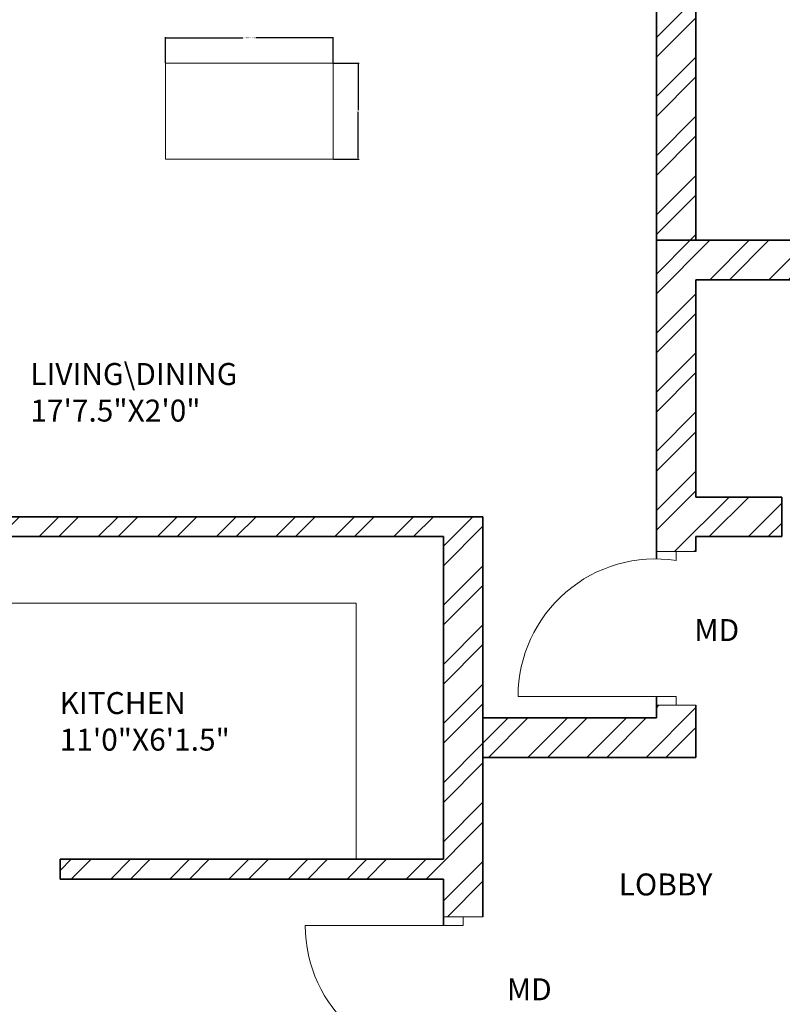
# Model space of a CAD drawing. Units: inches. Extents: x 2120 to 4013, y 1390 to 3019.
# Tile 32 of 59: x 2484 to 2657, y 1964 to 2188. Entities that reach past the tile are written whole.
import ezdxf

# ---------------------------------------------------------------- set-up
doc = ezdxf.new("R2010")
doc.units = ezdxf.units.IN
for name, color, linetype, lineweight in [('A-ANNO-DIMS', 2, 'Continuous', 18), ('A-ANNO-TEXT', 7, 'Continuous', 18), ('A-AREA-IDEN', 7, 'Continuous', 18), ('A-DOOR', 3, 'Continuous', 18), ('A-FLOR-CASE', 8, 'Continuous', 18), ('A-FURN', 8, 'Continuous', 13), ('A-WALL', 7, 'Continuous', 35), ('A-WALL-PATT', 252, 'Continuous', 13)]:
    doc.layers.add(name, color=color, linetype=linetype, lineweight=lineweight)
doc.styles.get("Standard").update_dxf_attribs({"font": 'arial.ttf'})
doc.dimstyles.get("Standard").update_dxf_attribs({"dimtxt": 0.18, "dimasz": 0.18, "dimexe": 0.18, "dimexo": 0.0625, "dimgap": 0.09, "dimtad": 0, "dimtih": 1, "dimtoh": 1, "dimdec": 4, "dimzin": 0, "dimdsep": 46, "dimtxsty": 'Standard', "dimcen": 0.09, "dimadec": 0, "dimazin": 0, "dimtfac": 1, "dimtdec": 4, "dimtofl": 0, "dimtmove": 0, "dimatfit": 3, "dimfxl": 1, "dimtolj": 1, "dimtzin": 0, "dimarcsym": 0})

# ---------------------------------------------------------------- blocks, each defined once
blk = doc.blocks.new('DOOR-SWING-36IN-98p95DEG')
for p, q in [((31.5, 34.77), (40.5, 34.77)), ((40.5, 34.77), (36, 34.77)), ((36, 34.77), (36, 32.77)), ((36, 32.77), (0, 32.77)), ((31.5, 0), (40.5, 0)), ((36, 0), (36, 2)), ((40.5, 0), (36, 0))]:
    blk.add_line(p, q)
blk.add_arc((31.15, 32.77), 31.15, 180, 278.9496)
blk = doc.blocks.new('DOOR-SWING-36IN-98p61DEG')
for p, q in [((40.5, 34.96), (31.5, 34.96)), ((31.5, 34.96), (36, 34.96)), ((36, 34.96), (36, 32.96)), ((36, 2), (0, 2)), ((31.5, 0), (40.5, 0)), ((36, 0), (36, 2)), ((40.5, 0), (36, 0))]:
    blk.add_line(p, q)
blk.add_arc((31.31, 2), 31.31, 81.386, 180)
blk = doc.blocks.new('TABLE-COFFEE')
blk.add_lwpolyline([(0, 38.19), (21.88, 38.19), (21.88, 0), (0, 0)], close=True)
blk = doc.blocks.new('*D77')
at = {"layer": 'A-ANNO-DIMS', "color": 0, "lineweight": -2, "transparency": 16777216}
for p, q in [((2516.9, 2178.46), (2516.9, 2184.3)), ((2517.08, 2184.12), (2534.49, 2184.12)), ((2554.91, 2184.12), (2537.5, 2184.12)), ((2555.09, 2178.46), (2555.09, 2184.3))]:
    blk.add_line(p, q, dxfattribs=at)
at = {"layer": 'A-ANNO-DIMS', "color": 0, "transparency": 16777216}
for points in [[(2517.08, 2184.15), (2517.08, 2184.09), (2516.9, 2184.12)], [(2554.91, 2184.15), (2554.91, 2184.09), (2555.09, 2184.12)]]:
    blk.add_solid(points, dxfattribs=at)
at = {"layer": 'Defpoints', "color": 0, "transparency": 16777216}
for p in [(2516.9, 2184.12), (2516.9, 2178.4), (2555.09, 2178.4)]:
    blk.add_point(p, dxfattribs=at)
at = {"layer": 'A-ANNO-DIMS', "color": 0, "transparency": 16777216, "insert": (2535.99, 2184.12), "char_height": 0.18, "attachment_point": 5}
blk.add_mtext('\\A1;COFFEE TABLE 38 TYP.', dxfattribs=at)
blk = doc.blocks.new('*D78')
at = {"layer": 'A-ANNO-DIMS', "color": 0, "lineweight": -2, "transparency": 16777216}
for p, q in [((2555.15, 2178.4), (2561, 2178.4)), ((2560.82, 2178.22), (2560.82, 2167.64)), ((2560.82, 2156.7), (2560.82, 2167.28)), ((2555.15, 2156.52), (2561, 2156.52))]:
    blk.add_line(p, q, dxfattribs=at)
at = {"layer": 'A-ANNO-DIMS', "color": 0, "transparency": 16777216}
for points in [[(2560.79, 2178.22), (2560.85, 2178.22), (2560.82, 2178.4)], [(2560.79, 2156.7), (2560.85, 2156.7), (2560.82, 2156.52)]]:
    blk.add_solid(points, dxfattribs=at)
at = {"layer": 'Defpoints', "color": 0, "transparency": 16777216}
for p in [(2555.09, 2178.4), (2560.82, 2178.4), (2555.09, 2156.52)]:
    blk.add_point(p, dxfattribs=at)
at = {"layer": 'A-ANNO-DIMS', "color": 0, "transparency": 16777216, "insert": (2560.82, 2167.46), "char_height": 0.18, "attachment_point": 5}
blk.add_mtext('\\A1;22 TYP.', dxfattribs=at)

msp = doc.modelspace()

# ---------------------------------------------------------------- hatches: boundary and pattern name
at = {"layer": 'A-WALL-PATT'}
h = msp.add_hatch(dxfattribs=at)
h.set_pattern_fill('ANSI32', color=256)
h.paths.add_polyline_path([(2271.7331, 2343.531), (2283.3788, 2343.531), (2283.3788, 2348.031), (2283.3788, 2352.5306), (2262.7331, 2352.5306), (2262.7331, 2182.638), (2267.2331, 2182.638), (2271.7331, 2182.638), (2271.7331, 2219.031), (2391.7331, 2219.031), (2391.7331, 2214.189), (2393.9831, 2214.189), (2396.2331, 2214.189), (2396.2331, 2219.031), (2420.2331, 2219.031), (2420.2331, 2225.7535), (2417.2197, 2225.7535), (2415.7331, 2225.7535), (2415.7331, 2223.5306), (2271.7331, 2223.5306)])
h.paths.add_polyline_path([(2380.0942, 2352.5306), (2343.3788, 2352.5306), (2343.3788, 2343.531), (2363.2331, 2343.531), (2363.2331, 2288.8489), (2365.4831, 2288.8489), (2367.7331, 2288.8489), (2367.7331, 2343.531), (2380.0942, 2343.531)], flags=17)
h.paths.add_polyline_path([(2432.4339, 2352.5306), (2404.0943, 2352.5306), (2404.0943, 2343.531), (2415.7331, 2343.531), (2415.7331, 2264.0306), (2367.7331, 2264.0306), (2367.7331, 2266.4872), (2363.2331, 2266.4872), (2363.2331, 2259.531), (2367.7331, 2259.531), (2415.7331, 2259.531), (2415.7331, 2255.0658), (2420.2331, 2255.0658), (2420.2331, 2259.531), (2424.5717, 2259.531), (2424.5717, 2261.781), (2424.5717, 2264.0306), (2420.2331, 2264.0306), (2420.2331, 2343.531), (2432.4339, 2343.531)])
h.paths.add_polyline_path([(2508.9115, 2352.5306), (2456.4339, 2352.5306), (2456.4339, 2343.531), (2468.2331, 2343.531), (2468.2331, 2264.0306), (2448.0487, 2264.0306), (2448.0487, 2259.531), (2468.2331, 2259.531), (2468.2331, 2255.5496), (2472.7331, 2255.5496), (2472.7331, 2343.531), (2508.9115, 2343.531)])
h.paths.add_polyline_path([(2637.7331, 2352.5306), (2544.9116, 2352.5306), (2544.9116, 2343.531), (2589.7331, 2343.531), (2633.2331, 2343.531), (2637.7331, 2343.531)])
h.paths.add_polyline_path([(2594.2331, 2343.5306), (2589.7331, 2343.5306), (2589.7331, 2259.5306), (2589.7331, 2252.4915), (2591.9831, 2252.4915), (2594.2331, 2252.4915)])
h.paths.add_polyline_path([(2637.7331, 2223.5306), (2594.2331, 2223.5306), (2594.2331, 2230.1988), (2591.9831, 2230.1988), (2589.7331, 2230.1988), (2589.7331, 2223.5306), (2472.7331, 2223.5306), (2468.2331, 2223.5306), (2468.2331, 2219.031), (2628.7331, 2219.031), (2628.7331, 2138.031), (2637.7331, 2138.031)])
h.paths.add_polyline_path([(3822.6535, 2458.4402), (3874.9468, 2458.4402), (3874.9468, 2476.9866), (3822.6535, 2476.9866)], flags=9)
h.paths.add_polyline_path([(3834.6921, 2781.8174), (3935.9206, 2781.8174), (3935.9206, 2800.3638), (3834.6921, 2800.3638)], flags=9)
h.paths.add_polyline_path([(3832.2843, 2837.9683), (3884.5776, 2837.9683), (3884.5776, 2856.5146), (3832.2843, 2856.5146)], flags=9)
h.paths.add_polyline_path([(3830.9388, 2861.4782), (3956.8958, 2861.4782), (3956.8958, 2880.0245), (3830.9388, 2880.0245)], flags=9)
h.paths.add_polyline_path([(3870.6966, 2352.5752), (3887.9272, 2352.5752), (3887.9272, 2377.3037), (3870.6966, 2377.3037)], flags=9)
h.paths.add_polyline_path([(3289.2701, 2413.161), (3435.2223, 2413.161), (3435.2223, 2450.2538), (3289.2701, 2450.2538)], flags=9)
h.paths.add_polyline_path([(2487.6944, 2414.3601), (2637.8335, 2414.3601), (2637.8335, 2451.4528), (2487.6944, 2451.4528)], flags=9)
h.paths.add_polyline_path([(2567.3724, 1457.9199), (2815.296, 1457.9199), (2815.296, 1495.0127), (2567.3724, 1495.0127)], flags=9)
h.paths.add_polyline_path([(2655.3825, 2093.2363), (2685.9555, 2093.2363), (2685.9555, 2111.8937), (2655.3825, 2111.8937)], flags=9)
h.paths.add_polyline_path([(2543.9218, 1550.6671), (2587.8406, 1550.6671), (2587.8406, 1569.3244), (2543.9218, 1569.3244)], flags=9)
h.paths.add_polyline_path([(2905.1384, 1543.8113), (2949.0572, 1543.8113), (2949.0572, 1562.4686), (2905.1384, 1562.4686)], flags=9)
h.paths.add_polyline_path([(2736.4118, 1702.4736), (2784.2153, 1702.4736), (2784.2153, 1721.1309), (2736.4118, 1721.1309)], flags=9)
h.paths.add_polyline_path([(2912.8666, 1710.4168), (2951.707, 1710.4168), (2951.707, 1729.0741), (2912.8666, 1729.0741)], flags=9)
h.paths.add_polyline_path([(2923.5785, 1763.5038), (2959.7279, 1763.5038), (2959.7279, 1782.1611), (2923.5785, 1782.1611)], flags=9)
h.paths.add_polyline_path([(2925.2114, 1809.6137), (2967.1861, 1809.6137), (2967.1861, 1828.271), (2925.2114, 1828.271)], flags=9)
h.paths.add_polyline_path([(2996.2711, 1878.9003), (2996.2711, 1913.109), (2977.6138, 1913.109), (2977.6138, 1878.9003)], flags=9)
h.paths.add_polyline_path([(2883.0859, 1895.7192), (2927.1855, 1895.7192), (2927.1855, 1914.3766), (2883.0859, 1914.3766)], flags=9)
h.paths.add_polyline_path([(2787.3924, 1810.8013), (2841.0213, 1810.8013), (2841.0213, 1829.4587), (2787.3924, 1829.4587)], flags=9)
h.paths.add_polyline_path([(2775.6399, 2101.7395), (2829.2689, 2101.7395), (2829.2689, 2120.3968), (2775.6399, 2120.3968)], flags=9)
h.paths.add_polyline_path([(2913.0263, 2075.817), (2951.8667, 2075.817), (2951.8667, 2094.4744), (2913.0263, 2094.4744)], flags=9)
h.paths.add_polyline_path([(2929.966, 2133.3669), (2966.1154, 2133.3669), (2966.1154, 2152.0243), (2929.966, 2152.0243)], flags=9)
h.paths.add_polyline_path([(2932.7502, 2182.6088), (2968.8996, 2182.6088), (2968.8996, 2201.2662), (2932.7502, 2201.2662)], flags=9)
h.paths.add_polyline_path([(2996.0681, 2266.3173), (2996.0681, 2300.5261), (2977.4108, 2300.5261), (2977.4108, 2266.3173)], flags=9)
h.paths.add_polyline_path([(2885.1039, 2279.2186), (2929.2035, 2279.2186), (2929.2035, 2297.8759), (2885.1039, 2297.8759)], flags=9)
h.paths.add_polyline_path([(2735.7042, 2218.3197), (2783.5078, 2218.3197), (2783.5078, 2236.9771), (2735.7042, 2236.9771)], flags=9)
h.paths.add_polyline_path([(2635.6049, 2044.0085), (2648.9678, 2044.0085), (2648.9678, 2054.312), (2635.6049, 2054.312)], flags=9)
h.paths.add_polyline_path([(2714.0148, 1923.0473), (2727.3777, 1923.0473), (2727.3777, 1933.3508), (2714.0148, 1933.3508)], flags=9)
h.paths.add_polyline_path([(2709.0345, 1988.1628), (2722.3974, 1988.1628), (2722.3974, 1998.4663), (2709.0345, 1998.4663)], flags=9)
h.paths.add_polyline_path([(2592.8935, 1962.1763), (2606.2564, 1962.1763), (2606.2564, 1972.4799), (2592.8935, 1972.4799)], flags=9)
h.paths.add_polyline_path([(2618.3996, 1985.9724), (2644.1942, 1985.9724), (2644.1942, 1996.2759), (2618.3996, 1996.2759)], flags=9)
h.paths.add_polyline_path([(2601.279, 1920.5869), (2614.6419, 1920.5869), (2614.6419, 1930.8904), (2601.279, 1930.8904)], flags=9)
h.paths.add_polyline_path([(2692.3278, 1932.7645), (2704.5311, 1932.7645), (2704.5311, 1943.0681), (2692.3278, 1943.0681)], flags=9)
h.paths.add_polyline_path([(2311.122, 1672.7318), (2355.0408, 1672.7318), (2355.0408, 1691.3892), (2311.122, 1691.3892)], flags=9)
h.paths.add_polyline_path([(2456.2551, 1632.3198), (2492.4796, 1632.3198), (2492.4796, 1650.9772), (2456.2551, 1650.9772)], flags=9)
h.paths.add_polyline_path([(2401.0766, 1631.4793), (2437.301, 1631.4793), (2437.301, 1650.1367), (2401.0766, 1650.1367)], flags=9)
h.paths.add_polyline_path([(2546.7054, 1700.9235), (2594.509, 1700.9235), (2594.509, 1719.5809), (2546.7054, 1719.5809)], flags=9)
h.paths.add_polyline_path([(2445.4866, 1766.9937), (2497.5261, 1766.9937), (2497.5261, 1785.651), (2445.4866, 1785.651)], flags=9)
h.paths.add_polyline_path([(2287.9992, 1739.7675), (2326.8396, 1739.7675), (2326.8396, 1758.4248), (2287.9992, 1758.4248)], flags=9)
h.paths.add_polyline_path([(2458.5279, 1924.7607), (2510.5675, 1924.7607), (2510.5675, 1943.4181), (2458.5279, 1943.4181)], flags=9)
h.paths.add_polyline_path([(2309.2811, 1902.7642), (2345.4305, 1902.7642), (2345.4305, 1921.4215), (2309.2811, 1921.4215)], flags=9)
h.paths.add_polyline_path([(2490.7554, 2018.9392), (2530.7896, 2018.9392), (2530.7896, 2037.5965), (2490.7554, 2037.5965)], flags=9)
h.paths.add_polyline_path([(2402.143, 2024.7393), (2438.5414, 2024.7393), (2438.5414, 2043.3966), (2402.143, 2043.3966)], flags=9)
h.paths.add_polyline_path([(2287.856, 1931.7926), (2326.6964, 1931.7926), (2326.6964, 1950.4499), (2287.856, 1950.4499)], flags=9)
h.paths.add_polyline_path([(2281.7979, 2193.5771), (2320.6383, 2193.5771), (2320.6383, 2212.2344), (2281.7979, 2212.2344)], flags=25)
h.paths.add_polyline_path([(2484.0754, 2093.892), (2536.115, 2093.892), (2536.115, 2112.5494), (2484.0754, 2112.5494)], flags=9)
h.paths.add_polyline_path([(2624.7948, 2281.8639), (2624.7948, 2311.4137), (2606.1375, 2311.4137), (2606.1375, 2281.8639)], flags=9)
h.paths.add_polyline_path([(2507.5036, 2290.3639), (2541.934, 2290.3639), (2541.934, 2309.0212), (2507.5036, 2309.0212)], flags=9)
h.paths.add_polyline_path([(2423.1076, 2285.2202), (2459.332, 2285.2202), (2459.332, 2303.8776), (2423.1076, 2303.8776)], flags=9)
h.paths.add_polyline_path([(2374.5467, 2289.6272), (2410.7711, 2289.6272), (2410.7711, 2308.2846), (2374.5467, 2308.2846)], flags=25)
h.paths.add_polyline_path([(2277.4907, 2227.5651), (2316.3311, 2227.5651), (2316.3311, 2246.2224), (2277.4907, 2246.2224)], flags=25)
h.paths.add_polyline_path([(2655.3825, 2093.2367), (2685.9555, 2093.2367), (2685.9555, 2111.894), (2655.3825, 2111.894)], flags=9)
h.paths.add_polyline_path([(2543.9217, 1550.6674), (2587.8406, 1550.6674), (2587.8406, 1569.3247), (2543.9217, 1569.3247)], flags=9)
h.paths.add_polyline_path([(2905.1384, 1543.8116), (2949.0572, 1543.8116), (2949.0572, 1562.4689), (2905.1384, 1562.4689)], flags=9)
h.paths.add_polyline_path([(2736.4118, 1702.4739), (2784.2153, 1702.4739), (2784.2153, 1721.1312), (2736.4118, 1721.1312)], flags=9)
h.paths.add_polyline_path([(2912.8666, 1710.4171), (2951.707, 1710.4171), (2951.707, 1729.0744), (2912.8666, 1729.0744)], flags=9)
h.paths.add_polyline_path([(2923.5785, 1763.5041), (2959.7279, 1763.5041), (2959.7279, 1782.1614), (2923.5785, 1782.1614)], flags=9)
h.paths.add_polyline_path([(2925.2114, 1809.614), (2967.1861, 1809.614), (2967.1861, 1828.2713), (2925.2114, 1828.2713)], flags=9)
h.paths.add_polyline_path([(2996.2711, 1878.9006), (2996.2711, 1913.1094), (2977.6137, 1913.1094), (2977.6137, 1878.9006)], flags=9)
h.paths.add_polyline_path([(2883.0859, 1895.7195), (2927.1855, 1895.7195), (2927.1855, 1914.3769), (2883.0859, 1914.3769)], flags=9)
h.paths.add_polyline_path([(2787.3924, 1810.8016), (2841.0213, 1810.8016), (2841.0213, 1829.459), (2787.3924, 1829.459)], flags=9)
h.paths.add_polyline_path([(2775.6399, 2101.7398), (2829.2688, 2101.7398), (2829.2688, 2120.3971), (2775.6399, 2120.3971)], flags=9)
h.paths.add_polyline_path([(2913.0263, 2075.8173), (2951.8667, 2075.8173), (2951.8667, 2094.4747), (2913.0263, 2094.4747)], flags=9)
h.paths.add_polyline_path([(2929.966, 2133.3672), (2966.1154, 2133.3672), (2966.1154, 2152.0246), (2929.966, 2152.0246)], flags=9)
h.paths.add_polyline_path([(2932.7502, 2182.6091), (2968.8996, 2182.6091), (2968.8996, 2201.2665), (2932.7502, 2201.2665)], flags=9)
h.paths.add_polyline_path([(2996.0681, 2266.3176), (2996.0681, 2300.5264), (2977.4108, 2300.5264), (2977.4108, 2266.3176)], flags=9)
h.paths.add_polyline_path([(2885.1039, 2279.2189), (2929.2035, 2279.2189), (2929.2035, 2297.8762), (2885.1039, 2297.8762)], flags=9)
h.paths.add_polyline_path([(2735.7042, 2218.32), (2783.5078, 2218.32), (2783.5078, 2236.9774), (2735.7042, 2236.9774)], flags=9)
h.paths.add_polyline_path([(2635.6048, 2044.0088), (2648.9677, 2044.0088), (2648.9677, 2054.3123), (2635.6048, 2054.3123)], flags=9)
h.paths.add_polyline_path([(2714.0148, 1923.0476), (2727.3777, 1923.0476), (2727.3777, 1933.3511), (2714.0148, 1933.3511)], flags=9)
h.paths.add_polyline_path([(2709.0345, 1988.1631), (2722.3974, 1988.1631), (2722.3974, 1998.4666), (2709.0345, 1998.4666)], flags=9)
h.paths.add_polyline_path([(2592.8935, 1962.1766), (2606.2564, 1962.1766), (2606.2564, 1972.4802), (2592.8935, 1972.4802)], flags=9)
h.paths.add_polyline_path([(2618.3995, 1985.9727), (2644.1942, 1985.9727), (2644.1942, 1996.2762), (2618.3995, 1996.2762)], flags=9)
h.paths.add_polyline_path([(2601.279, 1920.5872), (2614.6419, 1920.5872), (2614.6419, 1930.8908), (2601.279, 1930.8908)], flags=9)
h.paths.add_polyline_path([(2692.3278, 1932.7648), (2704.5311, 1932.7648), (2704.5311, 1943.0684), (2692.3278, 1943.0684)], flags=9)
h.paths.add_polyline_path([(2311.122, 1672.7321), (2355.0408, 1672.7321), (2355.0408, 1691.3895), (2311.122, 1691.3895)], flags=9)
h.paths.add_polyline_path([(2456.2551, 1632.3201), (2492.4795, 1632.3201), (2492.4795, 1650.9775), (2456.2551, 1650.9775)], flags=9)
h.paths.add_polyline_path([(2401.0766, 1631.4796), (2437.301, 1631.4796), (2437.301, 1650.137), (2401.0766, 1650.137)], flags=9)
h.paths.add_polyline_path([(2546.7054, 1700.9238), (2594.509, 1700.9238), (2594.509, 1719.5812), (2546.7054, 1719.5812)], flags=9)
h.paths.add_polyline_path([(2445.4866, 1766.994), (2497.5261, 1766.994), (2497.5261, 1785.6513), (2445.4866, 1785.6513)], flags=9)
h.paths.add_polyline_path([(2287.9992, 1739.7678), (2326.8396, 1739.7678), (2326.8396, 1758.4251), (2287.9992, 1758.4251)], flags=9)
h.paths.add_polyline_path([(2458.5279, 1924.7611), (2510.5675, 1924.7611), (2510.5675, 1943.4184), (2458.5279, 1943.4184)], flags=9)
h.paths.add_polyline_path([(2309.2811, 1902.7645), (2345.4305, 1902.7645), (2345.4305, 1921.4218), (2309.2811, 1921.4218)], flags=9)
h.paths.add_polyline_path([(2490.7554, 2018.9395), (2530.7895, 2018.9395), (2530.7895, 2037.5968), (2490.7554, 2037.5968)], flags=9)
h.paths.add_polyline_path([(2402.143, 2024.7396), (2438.5413, 2024.7396), (2438.5413, 2043.3969), (2402.143, 2043.3969)], flags=9)
h.paths.add_polyline_path([(2287.856, 1931.7929), (2326.6964, 1931.7929), (2326.6964, 1950.4502), (2287.856, 1950.4502)], flags=9)
h.paths.add_polyline_path([(2281.7979, 2193.5774), (2320.6383, 2193.5774), (2320.6383, 2212.2347), (2281.7979, 2212.2347)], flags=25)
h.paths.add_polyline_path([(2484.0754, 2093.8924), (2536.115, 2093.8924), (2536.115, 2112.5497), (2484.0754, 2112.5497)], flags=9)
h.paths.add_polyline_path([(2624.7948, 2281.8642), (2624.7948, 2311.414), (2606.1374, 2311.414), (2606.1374, 2281.8642)], flags=9)
h.paths.add_polyline_path([(2507.5035, 2290.3642), (2541.934, 2290.3642), (2541.934, 2309.0215), (2507.5035, 2309.0215)], flags=9)
h.paths.add_polyline_path([(2423.1075, 2285.2205), (2459.332, 2285.2205), (2459.332, 2303.8779), (2423.1075, 2303.8779)], flags=9)
h.paths.add_polyline_path([(2374.5467, 2289.6275), (2410.7711, 2289.6275), (2410.7711, 2308.2849), (2374.5467, 2308.2849)], flags=25)
h.paths.add_polyline_path([(2277.4907, 2227.5654), (2316.3311, 2227.5654), (2316.3311, 2246.2227), (2277.4907, 2246.2227)], flags=25)
h = msp.add_hatch(dxfattribs=at)
h.set_pattern_fill('ANSI32', color=256)
h.paths.add_polyline_path([(2271.7331, 1980.389), (2262.7331, 1980.389), (2262.7331, 1912.8434), (2267.2331, 1912.8434), (2271.7331, 1912.8434), (2271.7331, 1922.531), (2351.2331, 1922.531), (2351.2331, 1901.4728), (2355.7331, 1901.4728), (2355.7331, 1922.531), (2357.9815, 1922.531), (2357.9815, 1926.5306), (2271.7331, 1926.5306)])
h.paths.add_polyline_path([(2589.2331, 1949.1622), (2584.7331, 1949.1622), (2580.2331, 1949.1622), (2580.2331, 1874.5306), (2355.7331, 1874.5306), (2355.7331, 1880.1922), (2351.2331, 1880.1922), (2351.2331, 1874.5306), (2271.7331, 1874.5306), (2271.7331, 1888.8431), (2262.7331, 1888.8431), (2262.7331, 1842.2909), (2267.2331, 1842.2909), (2271.7331, 1842.2909), (2271.7331, 1865.531), (2415.7331, 1865.531), (2415.7331, 1779.7286), (2420.2331, 1779.7286), (2420.2331, 1865.531), (2589.2331, 1865.531)])
h.paths.add_polyline_path([(2271.7331, 1782.2906), (2262.7331, 1782.2906), (2262.7331, 1711.4639), (2267.2331, 1711.4639), (2271.7331, 1711.4639), (2271.7331, 1738.031), (2420.2331, 1738.031), (2420.2331, 1742.531), (2420.2331, 1747.3376), (2417.9831, 1747.3376), (2415.7331, 1747.3376), (2415.7331, 1742.5306), (2271.7331, 1742.5306)])
h.paths.add_polyline_path([(2271.7331, 1627.031), (2362.3957, 1627.031), (2362.3957, 1629.281), (2362.3957, 1631.5306), (2271.7331, 1631.5306), (2271.7331, 1675.4636), (2262.7331, 1675.4636), (2262.7331, 1581.531), (2405.3032, 1581.531), (2405.3032, 1586.031), (2405.3032, 1590.5306), (2396.2331, 1590.5306), (2396.2331, 1691.4513), (2418.7206, 1691.4513), (2418.7206, 1695.951), (2396.2331, 1695.951), (2391.7331, 1695.951), (2391.7331, 1631.5306), (2386.7425, 1631.5306), (2386.7425, 1629.2806), (2386.7425, 1627.031), (2391.7331, 1627.031), (2391.7331, 1586.1709), (2271.7331, 1586.1709)])
h.paths.add_polyline_path([(2459.6703, 1590.5306), (2429.3032, 1590.5306), (2429.3032, 1581.531), (2459.6703, 1581.531), (2459.6703, 1586.031)])
h.paths.add_polyline_path([(2501.2331, 1590.531), (2501.2331, 1665.0195), (2498.9831, 1665.0195), (2496.7331, 1665.0195), (2496.7331, 1590.5306), (2483.8201, 1590.5306), (2483.8201, 1590.1579), (2483.6704, 1590.1579), (2483.6704, 1581.531), (2505.0196, 1581.531), (2505.0196, 1583.781), (2505.0196, 1586.0306), (2501.2331, 1586.0306)])
h.paths.add_polyline_path([(2544.1361, 1583.781), (2544.1361, 1586.0306), (2527.1368, 1586.0306), (2527.1368, 1583.7806), (2527.1368, 1581.531), (2544.1361, 1581.531)])
h.paths.add_polyline_path([(3822.6535, 2458.4402), (3874.9468, 2458.4402), (3874.9468, 2476.9866), (3822.6535, 2476.9866)], flags=9)
h.paths.add_polyline_path([(3834.6921, 2781.8174), (3935.9206, 2781.8174), (3935.9206, 2800.3638), (3834.6921, 2800.3638)], flags=9)
h.paths.add_polyline_path([(3832.2843, 2837.9683), (3884.5776, 2837.9683), (3884.5776, 2856.5146), (3832.2843, 2856.5146)], flags=9)
h.paths.add_polyline_path([(3830.9388, 2861.4782), (3956.8958, 2861.4782), (3956.8958, 2880.0245), (3830.9388, 2880.0245)], flags=9)
h.paths.add_polyline_path([(3870.6966, 2352.5752), (3887.9272, 2352.5752), (3887.9272, 2377.3037), (3870.6966, 2377.3037)], flags=9)
h.paths.add_polyline_path([(3289.2701, 2413.161), (3435.2223, 2413.161), (3435.2223, 2450.2538), (3289.2701, 2450.2538)], flags=9)
h.paths.add_polyline_path([(2487.6944, 2414.3601), (2637.8335, 2414.3601), (2637.8335, 2451.4528), (2487.6944, 2451.4528)], flags=9)
h.paths.add_polyline_path([(2567.3724, 1457.9199), (2815.296, 1457.9199), (2815.296, 1495.0127), (2567.3724, 1495.0127)], flags=9)
h.paths.add_polyline_path([(2655.3825, 2093.2363), (2685.9555, 2093.2363), (2685.9555, 2111.8937), (2655.3825, 2111.8937)], flags=9)
h.paths.add_polyline_path([(2543.9218, 1550.6671), (2587.8406, 1550.6671), (2587.8406, 1569.3244), (2543.9218, 1569.3244)], flags=9)
h.paths.add_polyline_path([(2905.1384, 1543.8113), (2949.0572, 1543.8113), (2949.0572, 1562.4686), (2905.1384, 1562.4686)], flags=9)
h.paths.add_polyline_path([(2736.4118, 1702.4736), (2784.2153, 1702.4736), (2784.2153, 1721.1309), (2736.4118, 1721.1309)], flags=9)
h.paths.add_polyline_path([(2912.8666, 1710.4168), (2951.707, 1710.4168), (2951.707, 1729.0741), (2912.8666, 1729.0741)], flags=9)
h.paths.add_polyline_path([(2923.5785, 1763.5038), (2959.7279, 1763.5038), (2959.7279, 1782.1611), (2923.5785, 1782.1611)], flags=9)
h.paths.add_polyline_path([(2925.2114, 1809.6137), (2967.1861, 1809.6137), (2967.1861, 1828.271), (2925.2114, 1828.271)], flags=9)
h.paths.add_polyline_path([(2996.2711, 1878.9003), (2996.2711, 1913.109), (2977.6138, 1913.109), (2977.6138, 1878.9003)], flags=9)
h.paths.add_polyline_path([(2883.0859, 1895.7192), (2927.1855, 1895.7192), (2927.1855, 1914.3766), (2883.0859, 1914.3766)], flags=9)
h.paths.add_polyline_path([(2787.3924, 1810.8013), (2841.0213, 1810.8013), (2841.0213, 1829.4587), (2787.3924, 1829.4587)], flags=9)
h.paths.add_polyline_path([(2775.6399, 2101.7395), (2829.2689, 2101.7395), (2829.2689, 2120.3968), (2775.6399, 2120.3968)], flags=9)
h.paths.add_polyline_path([(2913.0263, 2075.817), (2951.8667, 2075.817), (2951.8667, 2094.4744), (2913.0263, 2094.4744)], flags=9)
h.paths.add_polyline_path([(2929.966, 2133.3669), (2966.1154, 2133.3669), (2966.1154, 2152.0243), (2929.966, 2152.0243)], flags=9)
h.paths.add_polyline_path([(2932.7502, 2182.6088), (2968.8996, 2182.6088), (2968.8996, 2201.2662), (2932.7502, 2201.2662)], flags=9)
h.paths.add_polyline_path([(2996.0681, 2266.3173), (2996.0681, 2300.5261), (2977.4108, 2300.5261), (2977.4108, 2266.3173)], flags=9)
h.paths.add_polyline_path([(2885.1039, 2279.2186), (2929.2035, 2279.2186), (2929.2035, 2297.8759), (2885.1039, 2297.8759)], flags=9)
h.paths.add_polyline_path([(2735.7042, 2218.3197), (2783.5078, 2218.3197), (2783.5078, 2236.9771), (2735.7042, 2236.9771)], flags=9)
h.paths.add_polyline_path([(2635.6049, 2044.0085), (2648.9678, 2044.0085), (2648.9678, 2054.312), (2635.6049, 2054.312)], flags=9)
h.paths.add_polyline_path([(2714.0148, 1923.0473), (2727.3777, 1923.0473), (2727.3777, 1933.3508), (2714.0148, 1933.3508)], flags=9)
h.paths.add_polyline_path([(2709.0345, 1988.1628), (2722.3974, 1988.1628), (2722.3974, 1998.4663), (2709.0345, 1998.4663)], flags=9)
h.paths.add_polyline_path([(2592.8935, 1962.1763), (2606.2564, 1962.1763), (2606.2564, 1972.4799), (2592.8935, 1972.4799)], flags=9)
h.paths.add_polyline_path([(2618.3996, 1985.9724), (2644.1942, 1985.9724), (2644.1942, 1996.2759), (2618.3996, 1996.2759)], flags=9)
h.paths.add_polyline_path([(2601.279, 1920.5869), (2614.6419, 1920.5869), (2614.6419, 1930.8904), (2601.279, 1930.8904)], flags=9)
h.paths.add_polyline_path([(2692.3278, 1932.7645), (2704.5311, 1932.7645), (2704.5311, 1943.0681), (2692.3278, 1943.0681)], flags=9)
h.paths.add_polyline_path([(2311.122, 1672.7318), (2355.0408, 1672.7318), (2355.0408, 1691.3892), (2311.122, 1691.3892)], flags=25)
h.paths.add_polyline_path([(2456.2551, 1632.3198), (2492.4796, 1632.3198), (2492.4796, 1650.9772), (2456.2551, 1650.9772)], flags=9)
h.paths.add_polyline_path([(2401.0766, 1631.4793), (2437.301, 1631.4793), (2437.301, 1650.1367), (2401.0766, 1650.1367)], flags=9)
h.paths.add_polyline_path([(2546.7054, 1700.9235), (2594.509, 1700.9235), (2594.509, 1719.5809), (2546.7054, 1719.5809)], flags=9)
h.paths.add_polyline_path([(2445.4866, 1766.9937), (2497.5261, 1766.9937), (2497.5261, 1785.651), (2445.4866, 1785.651)], flags=9)
h.paths.add_polyline_path([(2287.9992, 1739.7675), (2326.8396, 1739.7675), (2326.8396, 1758.4248), (2287.9992, 1758.4248)], flags=24)
h.paths.add_polyline_path([(2458.5279, 1924.7607), (2510.5675, 1924.7607), (2510.5675, 1943.4181), (2458.5279, 1943.4181)], flags=25)
h.paths.add_polyline_path([(2309.2811, 1902.7642), (2345.4305, 1902.7642), (2345.4305, 1921.4215), (2309.2811, 1921.4215)], flags=25)
h.paths.add_polyline_path([(2490.7554, 2018.9392), (2530.7896, 2018.9392), (2530.7896, 2037.5965), (2490.7554, 2037.5965)], flags=9)
h.paths.add_polyline_path([(2402.143, 2024.7393), (2438.5414, 2024.7393), (2438.5414, 2043.3966), (2402.143, 2043.3966)], flags=9)
h.paths.add_polyline_path([(2287.856, 1931.7926), (2326.6964, 1931.7926), (2326.6964, 1950.4499), (2287.856, 1950.4499)], flags=25)
h.paths.add_polyline_path([(2281.7979, 2193.5771), (2320.6383, 2193.5771), (2320.6383, 2212.2344), (2281.7979, 2212.2344)], flags=9)
h.paths.add_polyline_path([(2484.0754, 2093.892), (2536.115, 2093.892), (2536.115, 2112.5494), (2484.0754, 2112.5494)], flags=9)
h.paths.add_polyline_path([(2624.7948, 2281.8639), (2624.7948, 2311.4137), (2606.1375, 2311.4137), (2606.1375, 2281.8639)], flags=9)
h.paths.add_polyline_path([(2507.5036, 2290.3639), (2541.934, 2290.3639), (2541.934, 2309.0212), (2507.5036, 2309.0212)], flags=9)
h.paths.add_polyline_path([(2423.1076, 2285.2202), (2459.332, 2285.2202), (2459.332, 2303.8776), (2423.1076, 2303.8776)], flags=9)
h.paths.add_polyline_path([(2374.5467, 2289.6272), (2410.7711, 2289.6272), (2410.7711, 2308.2846), (2374.5467, 2308.2846)], flags=9)
h.paths.add_polyline_path([(2277.4907, 2227.5651), (2316.3311, 2227.5651), (2316.3311, 2246.2224), (2277.4907, 2246.2224)], flags=9)
h.paths.add_polyline_path([(2655.3825, 2093.2367), (2685.9555, 2093.2367), (2685.9555, 2111.894), (2655.3825, 2111.894)], flags=9)
h.paths.add_polyline_path([(2543.9217, 1550.6674), (2587.8406, 1550.6674), (2587.8406, 1569.3247), (2543.9217, 1569.3247)], flags=9)
h.paths.add_polyline_path([(2905.1384, 1543.8116), (2949.0572, 1543.8116), (2949.0572, 1562.4689), (2905.1384, 1562.4689)], flags=9)
h.paths.add_polyline_path([(2736.4118, 1702.4739), (2784.2153, 1702.4739), (2784.2153, 1721.1312), (2736.4118, 1721.1312)], flags=9)
h.paths.add_polyline_path([(2912.8666, 1710.4171), (2951.707, 1710.4171), (2951.707, 1729.0744), (2912.8666, 1729.0744)], flags=9)
h.paths.add_polyline_path([(2923.5785, 1763.5041), (2959.7279, 1763.5041), (2959.7279, 1782.1614), (2923.5785, 1782.1614)], flags=9)
h.paths.add_polyline_path([(2925.2114, 1809.614), (2967.1861, 1809.614), (2967.1861, 1828.2713), (2925.2114, 1828.2713)], flags=9)
h.paths.add_polyline_path([(2996.2711, 1878.9006), (2996.2711, 1913.1094), (2977.6137, 1913.1094), (2977.6137, 1878.9006)], flags=9)
h.paths.add_polyline_path([(2883.0859, 1895.7195), (2927.1855, 1895.7195), (2927.1855, 1914.3769), (2883.0859, 1914.3769)], flags=9)
h.paths.add_polyline_path([(2787.3924, 1810.8016), (2841.0213, 1810.8016), (2841.0213, 1829.459), (2787.3924, 1829.459)], flags=9)
h.paths.add_polyline_path([(2775.6399, 2101.7398), (2829.2688, 2101.7398), (2829.2688, 2120.3971), (2775.6399, 2120.3971)], flags=9)
h.paths.add_polyline_path([(2913.0263, 2075.8173), (2951.8667, 2075.8173), (2951.8667, 2094.4747), (2913.0263, 2094.4747)], flags=9)
h.paths.add_polyline_path([(2929.966, 2133.3672), (2966.1154, 2133.3672), (2966.1154, 2152.0246), (2929.966, 2152.0246)], flags=9)
h.paths.add_polyline_path([(2932.7502, 2182.6091), (2968.8996, 2182.6091), (2968.8996, 2201.2665), (2932.7502, 2201.2665)], flags=9)
h.paths.add_polyline_path([(2996.0681, 2266.3176), (2996.0681, 2300.5264), (2977.4108, 2300.5264), (2977.4108, 2266.3176)], flags=9)
h.paths.add_polyline_path([(2885.1039, 2279.2189), (2929.2035, 2279.2189), (2929.2035, 2297.8762), (2885.1039, 2297.8762)], flags=9)
h.paths.add_polyline_path([(2735.7042, 2218.32), (2783.5078, 2218.32), (2783.5078, 2236.9774), (2735.7042, 2236.9774)], flags=9)
h.paths.add_polyline_path([(2635.6048, 2044.0088), (2648.9677, 2044.0088), (2648.9677, 2054.3123), (2635.6048, 2054.3123)], flags=9)
h.paths.add_polyline_path([(2714.0148, 1923.0476), (2727.3777, 1923.0476), (2727.3777, 1933.3511), (2714.0148, 1933.3511)], flags=9)
h.paths.add_polyline_path([(2709.0345, 1988.1631), (2722.3974, 1988.1631), (2722.3974, 1998.4666), (2709.0345, 1998.4666)], flags=9)
h.paths.add_polyline_path([(2592.8935, 1962.1766), (2606.2564, 1962.1766), (2606.2564, 1972.4802), (2592.8935, 1972.4802)], flags=9)
h.paths.add_polyline_path([(2618.3995, 1985.9727), (2644.1942, 1985.9727), (2644.1942, 1996.2762), (2618.3995, 1996.2762)], flags=9)
h.paths.add_polyline_path([(2601.279, 1920.5872), (2614.6419, 1920.5872), (2614.6419, 1930.8908), (2601.279, 1930.8908)], flags=9)
h.paths.add_polyline_path([(2692.3278, 1932.7648), (2704.5311, 1932.7648), (2704.5311, 1943.0684), (2692.3278, 1943.0684)], flags=9)
h.paths.add_polyline_path([(2311.122, 1672.7321), (2355.0408, 1672.7321), (2355.0408, 1691.3895), (2311.122, 1691.3895)], flags=25)
h.paths.add_polyline_path([(2456.2551, 1632.3201), (2492.4795, 1632.3201), (2492.4795, 1650.9775), (2456.2551, 1650.9775)], flags=9)
h.paths.add_polyline_path([(2401.0766, 1631.4796), (2437.301, 1631.4796), (2437.301, 1650.137), (2401.0766, 1650.137)], flags=9)
h.paths.add_polyline_path([(2546.7054, 1700.9238), (2594.509, 1700.9238), (2594.509, 1719.5812), (2546.7054, 1719.5812)], flags=9)
h.paths.add_polyline_path([(2445.4866, 1766.994), (2497.5261, 1766.994), (2497.5261, 1785.6513), (2445.4866, 1785.6513)], flags=9)
h.paths.add_polyline_path([(2287.9992, 1739.7678), (2326.8396, 1739.7678), (2326.8396, 1758.4251), (2287.9992, 1758.4251)], flags=24)
h.paths.add_polyline_path([(2458.5279, 1924.7611), (2510.5675, 1924.7611), (2510.5675, 1943.4184), (2458.5279, 1943.4184)], flags=25)
h.paths.add_polyline_path([(2309.2811, 1902.7645), (2345.4305, 1902.7645), (2345.4305, 1921.4218), (2309.2811, 1921.4218)], flags=25)
h.paths.add_polyline_path([(2490.7554, 2018.9395), (2530.7895, 2018.9395), (2530.7895, 2037.5968), (2490.7554, 2037.5968)], flags=9)
h.paths.add_polyline_path([(2402.143, 2024.7396), (2438.5413, 2024.7396), (2438.5413, 2043.3969), (2402.143, 2043.3969)], flags=9)
h.paths.add_polyline_path([(2287.856, 1931.7929), (2326.6964, 1931.7929), (2326.6964, 1950.4502), (2287.856, 1950.4502)], flags=25)
h.paths.add_polyline_path([(2281.7979, 2193.5774), (2320.6383, 2193.5774), (2320.6383, 2212.2347), (2281.7979, 2212.2347)], flags=9)
h.paths.add_polyline_path([(2484.0754, 2093.8924), (2536.115, 2093.8924), (2536.115, 2112.5497), (2484.0754, 2112.5497)], flags=9)
h.paths.add_polyline_path([(2624.7948, 2281.8642), (2624.7948, 2311.414), (2606.1374, 2311.414), (2606.1374, 2281.8642)], flags=9)
h.paths.add_polyline_path([(2507.5035, 2290.3642), (2541.934, 2290.3642), (2541.934, 2309.0215), (2507.5035, 2309.0215)], flags=9)
h.paths.add_polyline_path([(2423.1075, 2285.2205), (2459.332, 2285.2205), (2459.332, 2303.8779), (2423.1075, 2303.8779)], flags=9)
h.paths.add_polyline_path([(2374.5467, 2289.6275), (2410.7711, 2289.6275), (2410.7711, 2308.2849), (2374.5467, 2308.2849)], flags=9)
h.paths.add_polyline_path([(2277.4907, 2227.5654), (2316.3311, 2227.5654), (2316.3311, 2246.2227), (2277.4907, 2246.2227)], flags=9)
h = msp.add_hatch(dxfattribs=at)
h.set_pattern_fill('ANSI32', color=256)
h.paths.add_polyline_path([(2271.7331, 2122.6377), (2262.7331, 2122.6377), (2262.7331, 2040.3893), (2267.2331, 2040.3893), (2271.7331, 2040.3893), (2271.7331, 2044.8856), (2271.7331, 2070.531), (2391.7331, 2070.531), (2391.7331, 1926.5306), (2388.3993, 1926.5306), (2388.3993, 1922.531), (2395.7331, 1922.531), (2395.7331, 1992.531), (2400.4511, 1992.531), (2400.4511, 1997.0306), (2395.7331, 1997.0306), (2395.7331, 2070.531), (2443.7331, 2070.531), (2443.7331, 2046.1368), (2448.2331, 2046.1368), (2448.2331, 2070.531), (2580.2331, 2070.531), (2580.2331, 1997.0306), (2492.9076, 1997.0306), (2492.9076, 1992.531), (2580.2331, 1992.531), (2580.2331, 1983.9368), (2589.2331, 1983.9368), (2589.2331, 2070.531), (2589.2331, 2075.0306), (2396.2331, 2075.0306), (2396.2331, 2184.3565), (2393.9831, 2184.3565), (2391.7331, 2184.3565), (2391.7331, 2075.0306), (2271.7331, 2075.0306)])
h.paths.add_polyline_path([(2724.7331, 2138.0306), (2628.7331, 2138.0306), (2628.7331, 2070.5306), (2628.7331, 2067.0987), (2633.2331, 2067.0987), (2637.7331, 2067.0987), (2637.7331, 2070.531), (2657.3413, 2070.531), (2657.3413, 2079.5306), (2637.7331, 2079.5306), (2637.7331, 2129.031), (2715.7331, 2129.031), (2715.7331, 2079.5306), (2698.0378, 2079.5306), (2698.0378, 2070.531), (2715.7331, 2070.531), (2715.7331, 2012.1531), (2720.2331, 2012.1531), (2724.7331, 2012.1531)])
h.paths.add_polyline_path([(2724.7331, 2213.031), (2831.3209, 2213.031), (2831.3209, 2215.281), (2831.3209, 2217.5306), (2724.7331, 2217.5306), (2724.7331, 2343.531), (2751.8755, 2343.531), (2751.8755, 2352.5306), (2715.7331, 2352.5306), (2715.7331, 2138.031), (2724.7331, 2138.031)])
h.paths.add_polyline_path([(2902.53, 2352.5306), (2811.8755, 2352.5306), (2811.8755, 2343.531), (2867.2331, 2343.531), (2867.2331, 2217.5306), (2863.6364, 2217.5306), (2863.6364, 2213.031), (2871.7331, 2213.031), (2871.7331, 2217.531), (2871.7331, 2343.531), (2902.53, 2343.531)])
h.paths.add_polyline_path([(3009.7331, 2352.5306), (2938.53, 2352.5306), (2938.53, 2343.531), (2966.2331, 2343.531), (2966.2331, 2242.3281), (2968.4831, 2242.3281), (2970.7331, 2242.3281), (2970.7331, 2343.531), (3009.7331, 2343.531)])
h.paths.add_polyline_path([(3009.7331, 2217.5306), (2970.7331, 2217.5306), (2970.7331, 2220.5422), (2968.4831, 2220.5422), (2966.2331, 2220.5422), (2966.2331, 2217.5306), (2911.7752, 2217.5306), (2907.7331, 2217.5306), (2907.7331, 2213.0306), (2907.7331, 2194.9663), (2912.2331, 2194.9663), (2912.2331, 2213.031), (2970.7331, 2213.031), (3000.7331, 2213.031), (3000.7331, 2205.523), (3009.7331, 2205.523)])
h.paths.add_polyline_path([(3009.7331, 2181.5227), (3000.7331, 2181.5227), (3000.7331, 2165.0306), (2912.2331, 2165.0306), (2912.2331, 2170.8202), (2907.7331, 2170.8202), (2907.7331, 2165.0306), (2899.5169, 2165.0306), (2899.5169, 2162.7806), (2899.5169, 2160.531), (2907.7331, 2160.531), (2907.7331, 2137.3432), (2912.2331, 2137.3432), (2912.2331, 2160.531), (3000.7331, 2160.531), (3000.7331, 2150.4993), (3009.7331, 2150.4993)])
h.paths.add_polyline_path([(3009.7331, 2126.499), (3005.2331, 2126.499), (3000.7331, 2126.499), (3000.7331, 2112.5306), (2912.2331, 2112.5306), (2912.2331, 2115.6036), (2907.7331, 2115.6036), (2907.7331, 2108.031), (3000.7331, 2108.031), (3000.7331, 2084.7256), (3009.7331, 2084.7256)], flags=17)
h.paths.add_polyline_path([(3009.7331, 1971.531), (3009.7331, 2024.7253), (3000.7331, 2024.7253), (3000.7331, 2006.4153), (3000.7331, 1971.5306), (2864.2331, 1971.5306), (2864.2331, 2160.531), (2868.0522, 2160.531), (2868.0522, 2165.0306), (2859.7331, 2165.0306), (2859.7331, 1971.5306), (2724.7331, 1971.5306), (2724.7331, 1977.7012), (2715.7331, 1977.7012), (2715.7331, 1962.5306), (2715.7331, 1950.9035), (2720.2331, 1950.9035), (2724.7331, 1950.9035), (2724.7331, 1962.531), (2855.2331, 1962.531), (2859.7331, 1962.531), (2859.7331, 1835.031), (2864.2331, 1834.8158), (2864.2331, 1962.531), (2958.7331, 1962.531), (2958.7331, 1937.0925), (2963.2331, 1937.0925), (2963.2331, 1962.531), (3000.7331, 1962.531), (3009.7331, 1962.531)])
h.paths.add_polyline_path([(2724.7331, 1728.531), (2822.7164, 1728.531), (2822.7164, 1733.0306), (2724.7331, 1733.0306), (2724.7331, 1779.3416), (2715.7331, 1779.3416), (2715.7331, 1581.531), (2753.02, 1581.531), (2753.02, 1586.031), (2753.02, 1590.5306), (2724.7331, 1590.5306)])
h.paths.add_polyline_path([(2864.2331, 1590.531), (2864.2331, 1787.031), (2868.4075, 1787.031), (2868.4075, 1791.5306), (2859.7331, 1791.5306), (2859.7331, 1739.0306), (2859.7331, 1733.0306), (2854.3125, 1733.0306), (2854.3125, 1728.531), (2859.7331, 1728.531), (2859.7331, 1590.5306), (2813.02, 1590.5306), (2813.02, 1581.531), (2868.4123, 1581.531), (2868.4123, 1583.781), (2868.4123, 1586.0306), (2864.2331, 1586.0306)])
h.paths.add_polyline_path([(3009.7331, 1754.6619), (3000.7331, 1754.6619), (3000.7331, 1739.0306), (2912.2331, 1739.0306), (2912.2331, 1742.2257), (2907.7331, 1742.2257), (2907.7331, 1739.0306), (2907.7331, 1734.531), (3000.7331, 1734.531), (3000.7331, 1590.5306), (3000.7331, 1586.0306), (2971.3921, 1586.0306), (2971.3921, 1581.531), (3009.7331, 1581.531)])
h.paths.add_polyline_path([(2911.3921, 1583.781), (2911.3921, 1586.0306), (2891.2138, 1586.0306), (2891.2138, 1581.531), (2911.3921, 1581.531)])
h.paths.add_polyline_path([(3009.7331, 1799.8422), (3000.7331, 1799.8422), (3000.7331, 1791.5306), (2912.2331, 1791.5306), (2912.2331, 1796.3264), (2909.9831, 1796.3264), (2907.7331, 1796.3264), (2907.7331, 1791.5306), (2902.7033, 1791.5306), (2902.7033, 1787.031), (2907.7331, 1787.031), (2907.7331, 1761.1622), (2912.2331, 1761.1622), (2912.2331, 1787.031), (3000.7331, 1787.031), (3000.7331, 1778.6622), (3009.7331, 1778.6622)])
h.paths.add_polyline_path([(3009.7331, 1839.5306), (2963.2331, 1839.5306), (2963.2331, 1842.8629), (2960.9831, 1842.8629), (2958.7331, 1842.8629), (2958.7331, 1839.5306), (2907.7331, 1839.5306), (2907.7331, 1814.4599), (2912.2331, 1814.4599), (2912.2331, 1835.031), (3000.7331, 1835.031), (3000.7331, 1823.8425), (3009.7331, 1823.8425), (3009.7331, 1835.031)])
h.paths.add_polyline_path([(2963.2331, 1901.0922), (2960.9831, 1901.0922), (2958.7331, 1901.0922), (2958.7331, 1862.8843), (2963.2331, 1862.8843)], flags=17)
h.paths.add_polyline_path([(2724.7331, 1891.9826), (2724.7331, 1914.3416), (2715.7331, 1914.3416), (2715.7331, 1783.8416), (2637.7331, 1783.8416), (2637.7331, 1914.3416), (2628.7331, 1914.3416), (2624.7701, 1914.3416), (2624.7701, 1909.8416), (2624.7701, 1905.3419), (2628.7331, 1905.3419), (2628.7331, 1876.9915), (2628.7331, 1779.3419), (2637.7331, 1779.3419), (2715.7331, 1779.3419), (2724.7331, 1779.3419), (2724.7331, 1835.031)])
h.paths.add_polyline_path([(2637.7331, 1731.531), (2637.7331, 1779.3416), (2628.7331, 1779.3416), (2628.7331, 1731.5306), (2589.2331, 1731.5306), (2535.9814, 1731.5306), (2496.7331, 1731.5306), (2496.7331, 1725.6876), (2498.9831, 1725.6876), (2501.2331, 1725.6876), (2501.2331, 1727.031), (2628.7331, 1727.031), (2628.7331, 1680.4203), (2628.7331, 1590.5306), (2628.7331, 1586.0306), (2604.1361, 1586.0306), (2604.1361, 1581.531), (2637.7331, 1581.531), (2637.7331, 1590.531)])
h = msp.add_hatch(dxfattribs=at)
h.set_pattern_fill('ANSI32', color=256)
h.paths.add_polyline_path([(2637.7331, 2029.2261), (2637.7331, 2032.1412), (2633.2331, 2032.1412), (2628.7331, 2032.1412), (2628.7331, 2029.2258), (2589.2331, 2029.2258), (2589.2331, 2020.2261), (2637.7331, 2020.2261)])

# ---------------------------------------------------------------- linework, layer by layer
at = {"layer": 'A-FLOR-CASE'}
for p, q in [((2448.2331, 2055.3306), (2560.319, 2055.3306)), ((2448.2331, 2055.3303), (2560.319, 2055.3303)), ((2560.319, 2055.3306), (2560.319, 1997.031)), ((2560.319, 2055.3303), (2560.319, 1997.0306))]:
    msp.add_line(p, q, dxfattribs=at)
at = {"layer": 'A-WALL'}
for p, q in [((2637.7331, 2259.531), (2637.7331, 2138.031)), ((2637.7331, 2259.5306), (2637.7331, 2138.0306)), ((2628.7331, 2219.031), (2628.7331, 2138.031)), ((2628.7331, 2219.0306), (2628.7331, 2138.0306)), ((2628.7331, 2138.031), (2628.7331, 2070.531)), ((2724.7331, 2138.031), (2628.7331, 2138.031)), ((2628.7331, 2138.031), (2628.7331, 2070.531)), ((2628.7331, 2138.0306), (2628.7331, 2070.5306)), ((2628.7331, 2138.0306), (2628.7331, 2070.5306)), ((2724.7331, 2138.0306), (2628.7331, 2138.0306)), ((2637.7331, 2079.531), (2637.7331, 2129.031)), ((2637.7331, 2129.031), (2715.7331, 2129.031)), ((2637.7331, 2129.031), (2637.7331, 2079.531)), ((2637.7331, 2129.0306), (2637.7331, 2079.5306)), ((2637.7331, 2079.5306), (2637.7331, 2129.0306)), ((2637.7331, 2129.0306), (2715.7331, 2129.0306)), ((2657.3413, 2079.531), (2637.7331, 2079.531)), ((2657.3413, 2079.5306), (2637.7331, 2079.5306)), ((2657.3413, 2079.531), (2657.3413, 2070.531)), ((2657.3413, 2079.5306), (2657.3413, 2070.5306)), ((2396.2331, 2075.031), (2589.2331, 2075.031)), ((2396.2331, 2075.0306), (2589.2331, 2075.0306)), ((2589.2331, 2070.531), (2589.2331, 2075.031)), ((2589.2331, 2070.5306), (2589.2331, 2075.0306)), ((2448.2331, 2070.531), (2580.2331, 2070.531)), ((2448.2331, 2070.5306), (2580.2331, 2070.5306)), ((2580.2331, 2070.531), (2580.2331, 1997.031)), ((2580.2331, 2070.531), (2580.2331, 1997.031)), ((2580.2331, 2070.5306), (2580.2331, 1997.0306)), ((2580.2331, 2070.5306), (2580.2331, 1997.0306)), ((2589.2331, 2070.531), (2589.2331, 1983.9368)), ((2589.2331, 2070.5306), (2589.2331, 1983.9365)), ((2628.7331, 2065.4513), (2628.7331, 2070.531)), ((2628.7331, 2065.451), (2628.7331, 2070.5306)), ((2637.7331, 2070.531), (2657.3413, 2070.531)), ((2637.7331, 2070.531), (2637.7331, 2067.0987)), ((2637.7331, 2070.5306), (2657.3413, 2070.5306)), ((2637.7331, 2070.5306), (2637.7331, 2067.0984)), ((2628.7331, 2029.2261), (2628.7331, 2034.1415)), ((2628.7331, 2029.2258), (2628.7331, 2034.1412)), ((2637.7331, 2032.1415), (2637.7331, 2029.2261)), ((2637.7331, 2032.1412), (2637.7331, 2029.2258)), ((2628.7331, 2029.2261), (2589.2331, 2029.2261)), ((2628.7331, 2029.2258), (2589.2331, 2029.2258)), ((2637.7331, 2020.2261), (2637.7331, 2029.2261)), ((2637.7331, 2020.2258), (2637.7331, 2029.2258)), ((2589.2331, 2020.2261), (2637.7331, 2020.2261)), ((2589.2331, 2020.2258), (2637.7331, 2020.2258)), ((2580.2331, 1997.031), (2492.9076, 1997.031)), ((2492.9076, 1997.031), (2492.9076, 1992.531)), ((2580.2331, 1997.0306), (2492.9076, 1997.0306)), ((2492.9076, 1997.0306), (2492.9076, 1992.5306)), ((2492.9076, 1992.531), (2580.2331, 1992.531)), ((2492.9076, 1992.5306), (2580.2331, 1992.5306)), ((2580.2331, 1992.531), (2580.2331, 1981.9368)), ((2580.2331, 1992.5306), (2580.2331, 1981.9365))]:
    msp.add_line(p, q, dxfattribs=at)

# ---------------------------------------------------------------- block references
at = {"layer": 'A-DOOR'}
for name, p in [('DOOR-SWING-36IN-98p61DEG', (2597.2331, 2032.1415)), ('DOOR-SWING-36IN-98p61DEG', (2597.2331, 2032.1412)), ('DOOR-SWING-36IN-98p95DEG', (2548.7331, 1949.1625)), ('DOOR-SWING-36IN-98p95DEG', (2548.7331, 1949.1622))]:
    msp.add_blockref(name, p, dxfattribs=at)
at = {"layer": 'A-FURN'}
for p, rotation in [((2555.0905, 2156.5169), 90.00000000000207), ((2555.0905, 2156.5166), 90.00000000000122)]:
    msp.add_blockref('TABLE-COFFEE', p, dxfattribs=dict(at, rotation=rotation))

# ---------------------------------------------------------------- texts
at = {"layer": 'A-ANNO-TEXT', "char_height": 5, "attachment_point": 1}
for insert in [(2637.3733, 2051.739), (2637.3733, 2051.7387), (2594.6619, 1969.9069), (2594.6619, 1969.9065)]:
    msp.add_mtext_dynamic_manual_height_columns('MD', width=56.213303, gutter_width=12.5, heights=[0], dxfattribs=dict(at, insert=insert))
at = {"layer": 'A-AREA-IDEN', "char_height": 5, "attachment_point": 1}
for s, width, insert in [('LIVING\\\\DINING \\P17\'7.5"X2\'0"', 133.806403, (2486.086, 2110.0616)), ('LIVING\\\\DINING \\P17\'7.5"X2\'0"', 133.806403, (2486.086, 2110.0613)), ('KITCHEN\\P11\'0"X6\'1.5"', 166.862873, (2492.766, 2035.1087)), ('KITCHEN\\P11\'0"X6\'1.5"', 166.862873, (2492.766, 2035.1084)), ('LOBBY', 88.749226, (2620.1611, 1993.7916)), ('LOBBY', 88.749226, (2620.1611, 1993.7913))]:
    msp.add_mtext_dynamic_manual_height_columns(s, width=width, gutter_width=12.5, heights=[0], dxfattribs=dict(at, insert=insert))

# ---------------------------------------------------------------- dimensions: what is measured, and where the dimension line sits
at = {"layer": 'A-ANNO-DIMS'}
for base, p1, p2, angle, text, picture, middle in [((2516.8971, 2184.1249), (2555.0905, 2178.3959), (2516.8971, 2178.3959), 180, 'COFFEE TABLE <> TYP.', '*D77', (2535.9938, 2184.1249)), ((2560.8195, 2178.3959), (2555.0905, 2156.5169), (2555.0905, 2178.3959), 90, '<> TYP.', '*D78', (2560.8195, 2167.4564))]:
    dim = msp.add_linear_dim(base=base, p1=p1, p2=p2, angle=angle, text=text, dimstyle='Standard', override={"dimdec": 0, "dimlfac": 1, "dimrnd": 0, "dimzin": 0, "dimdsep": 46, "dimlunit": 2}, dxfattribs=at)
    dim.commit()
    dim.dimension.update_dxf_attribs({"geometry": picture, "text_midpoint": middle})

doc.saveas('drawing.dxf')
